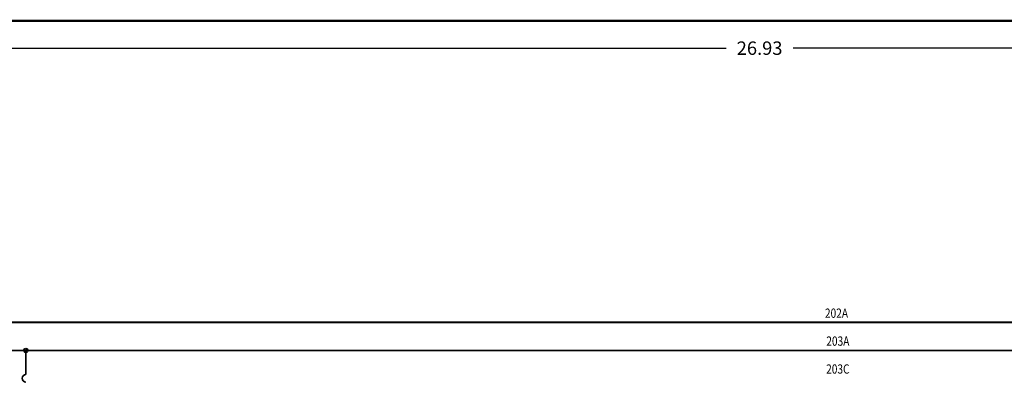
# Model space of a CAD drawing. Extents: x 0 to 33.5, y 0 to 22.4.
# Tile 5 of 8: x 6.7 to 19.9, y 17.7 to 22.4. Entities that reach past the tile are written whole.
import ezdxf
from ezdxf.enums import TextEntityAlignment as Align

# ---------------------------------------------------------------- set-up
doc = ezdxf.new("R2010")
doc.units = 0
doc.header["$MEASUREMENT"] = 0
for name, color, linetype, lineweight in [('A-ANNO-DIMS', 2, 'Continuous', 18), ('SYMS', 7, 'Continuous', 25), ('TITLE', 7, 'Continuous', 35), ('WIRENO', 72, 'Continuous', 18), ('WIRES', 7, 'Continuous', 35)]:
    doc.layers.add(name, color=color, linetype=linetype, lineweight=lineweight)
doc.styles.add('ITALIC', font='ITALIC')
doc.styles.add('SIMPLEX', font='SIMPLEX')
doc.styles.add('WD', font='romans.shx')
doc.dimstyles.get("Standard").update_dxf_attribs({"dimtxt": 0.18, "dimasz": 0.18, "dimexe": 0.18, "dimexo": 0.0625, "dimgap": 0.09, "dimtad": 0, "dimtih": 1, "dimtoh": 1, "dimdec": 4, "dimzin": 0, "dimdsep": 46, "dimtxsty": 'Standard', "dimcen": 0.09, "dimadec": 0, "dimazin": 0, "dimtfac": 1, "dimtdec": 4, "dimtofl": 0, "dimtmove": 0, "dimatfit": 3, "dimfxl": 1, "dimtolj": 1, "dimtzin": 0, "dimarcsym": 0})

# ---------------------------------------------------------------- blocks, each defined once
blk = doc.blocks.new('NO_NUM_acade_title')
at = {"layer": 'TITLE', "const_width": 0.0312}
blk.add_lwpolyline([(30.594, 0.281), (30.594, 22.177), (30.344, 22.427), (0.281, 22.427), (0.031, 22.177), (0.031, 0.281), (0.281, 0.031), (30.344, 0.031)], close=True, dxfattribs=at)
at = {"layer": 'TITLE', "style": 'ITALIC'}
for tag, height, p in [('TITLE#1', 0.125, (32.156, 3.406)), ('TITLE#2', 0.125, (32.156, 3.204)), ('TITLE#3', 0.125, (32.156, 3.001)), ('TITLE#4', 0.125, (32.156, 2.799)), ('DWG#', 0.2, (32.156, 0.826))]:
    blk.add_attdef(tag, text='', height=height, dxfattribs=at).set_placement(p, align=Align.CENTER)
at = {"layer": 'TITLE', "style": 'SIMPLEX'}
blk.add_attdef('CAD#', (30.826, 1.958), '', height=0.0938, rotation=90, dxfattribs=at)
at = {"layer": 'TITLE'}
for tag, p, height, style in [('JOB#', (31.464, 1.644), 0.0938, 'SIMPLEX'), ('SCALE', (31.353, 1.344), 0.0938, 'SIMPLEX'), ('DATE', (32.408, 1.344), 0.0938, 'SIMPLEX'), ('SHTS', (32.532, 0.25), 0.2, 'ITALIC')]:
    blk.add_attdef(tag, p, '', height=height, dxfattribs=dict(at, style=style))
at = {"layer": 'TITLE', "style": 'ITALIC'}
blk.add_attdef('SH#', text='', height=0.2, dxfattribs=at).set_placement((31.881, 0.25), align=Align.RIGHT)
at = {"layer": 'TITLE', "flags": 9}
blk.add_attdef('WD_TB', (31.219, 0.031), '', height=0.125, dxfattribs=at)
blk = doc.blocks.new('WDDOT')
for radius in [0.03, 0.0187, 0.00929]:
    blk.add_circle((0, 0), radius)
blk = doc.blocks.new('WD_WNH')
at = {"style": 'WD', "width": 0.8}
blk.add_attdef('WIRENO', text='', height=0.125, dxfattribs=at).set_placement((0, 0.062), align=Align.CENTER)
at = {"style": 'WD', "flags": 1}
for tag, p in [('W01USER', (0, 0.078)), ('W02USER', (0, 0.07)), ('W03USER', (0, 0.062)), ('W04USER', (0, 0.055)), ('W05USER', (0, 0.047)), ('W06USER', (0, 0.039)), ('W07USER', (0, 0.031)), ('W08USER', (0, 0.023)), ('W09USER', (0, 0.016)), ('W10USER', (0, 0.008))]:
    blk.add_attdef(tag, text='', height=0.005, dxfattribs=at).set_placement(p, align=Align.CENTER)
blk = doc.blocks.new('*D37')
at = {"layer": 'A-ANNO-DIMS', "color": 0, "lineweight": -2, "transparency": 16777216}
for p, q in [((3.125, 18.4375), (3.125, 22.239937)), ((30.05762, 18.46875), (30.05762, 22.239937)), ((3.305, 22.059937), (16.14131, 22.059937)), ((29.87762, 22.059937), (17.04131, 22.059937))]:
    blk.add_line(p, q, dxfattribs=at)
at = {"layer": 'A-ANNO-DIMS', "color": 0, "transparency": 16777216}
for points in [[(3.305, 22.089937), (3.305, 22.029937), (3.125, 22.059937)], [(29.87762, 22.089937), (29.87762, 22.029937), (30.05762, 22.059937)]]:
    blk.add_solid(points, dxfattribs=at)
at = {"layer": 'Defpoints', "color": 0, "transparency": 16777216}
for p in [(30.05762, 22.059937), (3.125, 18.375), (30.05762, 18.40625)]:
    blk.add_point(p, dxfattribs=at)
at = {"layer": 'A-ANNO-DIMS', "color": 0, "transparency": 16777216, "insert": (16.59131, 22.059937), "char_height": 0.18, "attachment_point": 5}
blk.add_mtext('\\A1;26.93', dxfattribs=at)
blk = doc.blocks.new('*D61')
at = {"layer": 'A-ANNO-DIMS', "color": 0, "lineweight": -2, "transparency": 16777216}
for p, q in [((23.088, 18.379), (1.48, 18.379)), ((1.66, 18.199), (1.66, 15.997)), ((1.66, 13.436), (1.66, 15.637)), ((20.838, 13.256), (1.48, 13.256))]:
    blk.add_line(p, q, dxfattribs=at)
at = {"layer": 'A-ANNO-DIMS', "color": 0, "transparency": 16777216}
for points in [[(1.63, 18.199), (1.69, 18.199), (1.66, 18.379)], [(1.63, 13.436), (1.69, 13.436), (1.66, 13.256)]]:
    blk.add_solid(points, dxfattribs=at)
at = {"layer": 'Defpoints', "color": 0, "transparency": 16777216}
for p in [(23.151, 18.379), (1.66, 13.256), (20.901, 13.256)]:
    blk.add_point(p, dxfattribs=at)
at = {"layer": 'A-ANNO-DIMS', "color": 0, "transparency": 16777216, "insert": (1.66, 15.817), "char_height": 0.18, "attachment_point": 5}
blk.add_mtext('\\A1;5.123', dxfattribs=at)

msp = doc.modelspace()

# ---------------------------------------------------------------- linework, layer by layer
at = {"layer": 'WIRES'}
for p, q in [((5.1875, 18.375), (30.0576, 18.375)), ((5.1875, 18), (30.0939, 18)), ((6.75, 18), (6.75, 17.675))]:
    msp.add_line(p, q, dxfattribs=at)
msp.add_arc((6.75, 17.625), 0.05, 90, 270, dxfattribs=at)

# ---------------------------------------------------------------- block references
at = {"layer": 'SYMS'}
msp.add_blockref('WDDOT', (6.75, 18), dxfattribs=at)
at = {"layer": 'TITLE'}
msp.add_blockref('NO_NUM_acade_title', (0, 0), dxfattribs=at)
at = {"layer": 'WIRENO'}
ref = msp.add_blockref('WD_WNH', (17.6226, 18.375), dxfattribs=at)
ref.add_attrib('WIRENO', '202A', dxfattribs={"linetype": 'Continuous', "height": 0.125, "style": 'WD', "width": 0.8}).set_placement((17.6226, 18.4375), align=Align.CENTER)
ref = msp.add_blockref('WD_WNH', (17.6407, 18), dxfattribs=at)
ref.add_attrib('WIRENO', '203A', dxfattribs={"linetype": 'Continuous', "height": 0.125, "style": 'WD', "width": 0.8}).set_placement((17.6407, 18.0625), align=Align.CENTER)
ref = msp.add_blockref('WD_WNH', (17.6407, 17.625), dxfattribs=at)
ref.add_attrib('WIRENO', '203C', dxfattribs={"linetype": 'Continuous', "height": 0.125, "style": 'WD', "width": 0.8}).set_placement((17.6407, 17.6875), align=Align.CENTER)

# ---------------------------------------------------------------- dimensions: what is measured, and where the dimension line sits
at = {"layer": 'A-ANNO-DIMS'}
dim = msp.add_linear_dim(base=(30.0576, 22.0599), p1=(3.125, 18.375), p2=(30.0576, 18.4062), dimstyle='Standard', override={"dimdec": 2, "dimlfac": 1, "dimrnd": 0, "dimzin": 0, "dimdsep": 46, "dimlunit": 2}, dxfattribs=at)
dim.commit()
dim.dimension.update_dxf_attribs({"geometry": '*D37', "text_midpoint": (16.5913, 22.0599)})
dim = msp.add_linear_dim(base=(1.66, 13.2558), p1=(23.151, 18.3786), p2=(20.9008, 13.2558), angle=90, dimstyle='Standard', override={"dimdec": 3, "dimlfac": 1, "dimrnd": 0, "dimzin": 0, "dimdsep": 46, "dimlunit": 2}, dxfattribs=at)
dim.commit()
dim.dimension.update_dxf_attribs({"geometry": '*D61', "text_midpoint": (1.66, 15.8172)})

doc.saveas('drawing.dxf')
